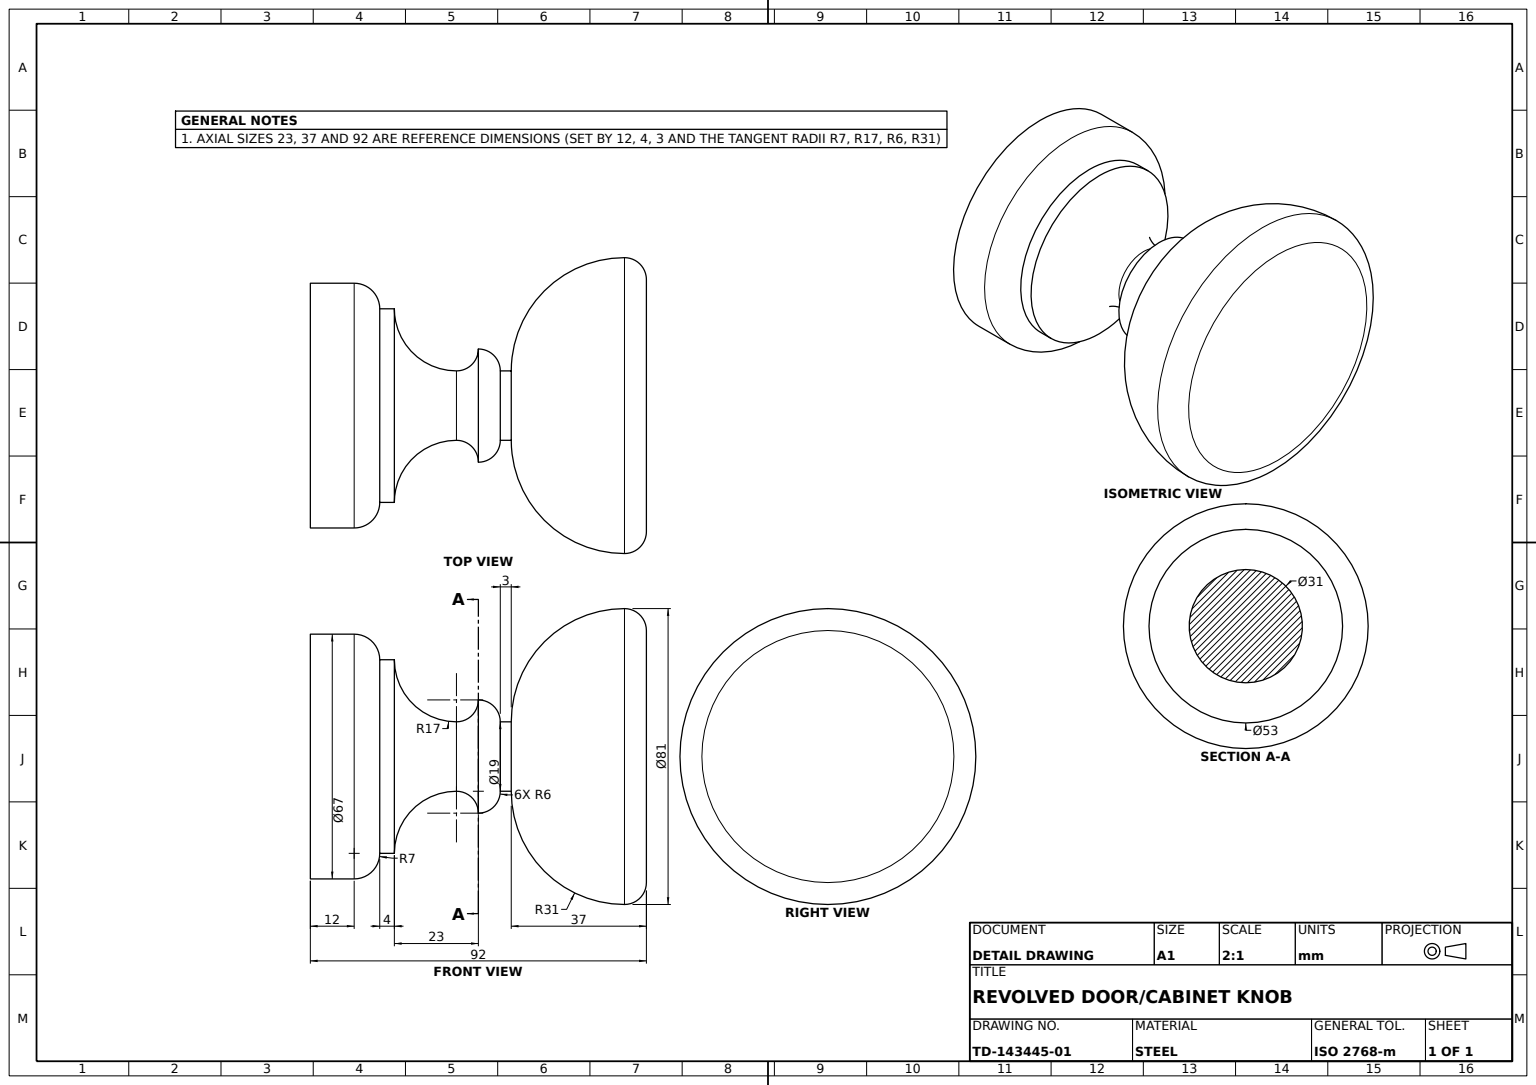
from build123d import *


with BuildPart() as part:
    # Knob Profile Sketch → Knob Body Revolve (revolve)
    with BuildSketch(Plane.XY, mode=Mode.PRIVATE) as knob_body_revolve_sk:
        with BuildLine():
            Line((0, 0), (33.5, 0))
            Line((33.5, 0), (33.5, 12))
            ThreePointArc((33.5, 12), (31.449747468, 16.949747468), (26.5, 19))
            Line((26.5, 19), (26.5, 23))
            ThreePointArc((26.5, 23), (14.47918472, 27.97918472), (9.5, 40))
            ThreePointArc((9.5, 40), (11.257359313, 44.242640687), (15.5, 46))
            ThreePointArc((15.5, 46), (13.742640687, 50.242640687), (9.5, 52))
            Line((9.5, 52), (9.5, 55))
            ThreePointArc((9.5, 55), (31.420310217, 64.079689783), (40.5, 86))
            ThreePointArc((40.5, 86), (38.742640687, 90.242640687), (34.5, 92))
            Line((34.5, 92), (0, 92))
            Line((0, 92), (0, 0))
        make_face()
    revolve(knob_body_revolve_sk.sketch.rotate(Axis((0, 92, 0), (0, -1, 0)), 180), axis=Axis((0, 92, 0), (0, -1, 0)))


solid = part.part
